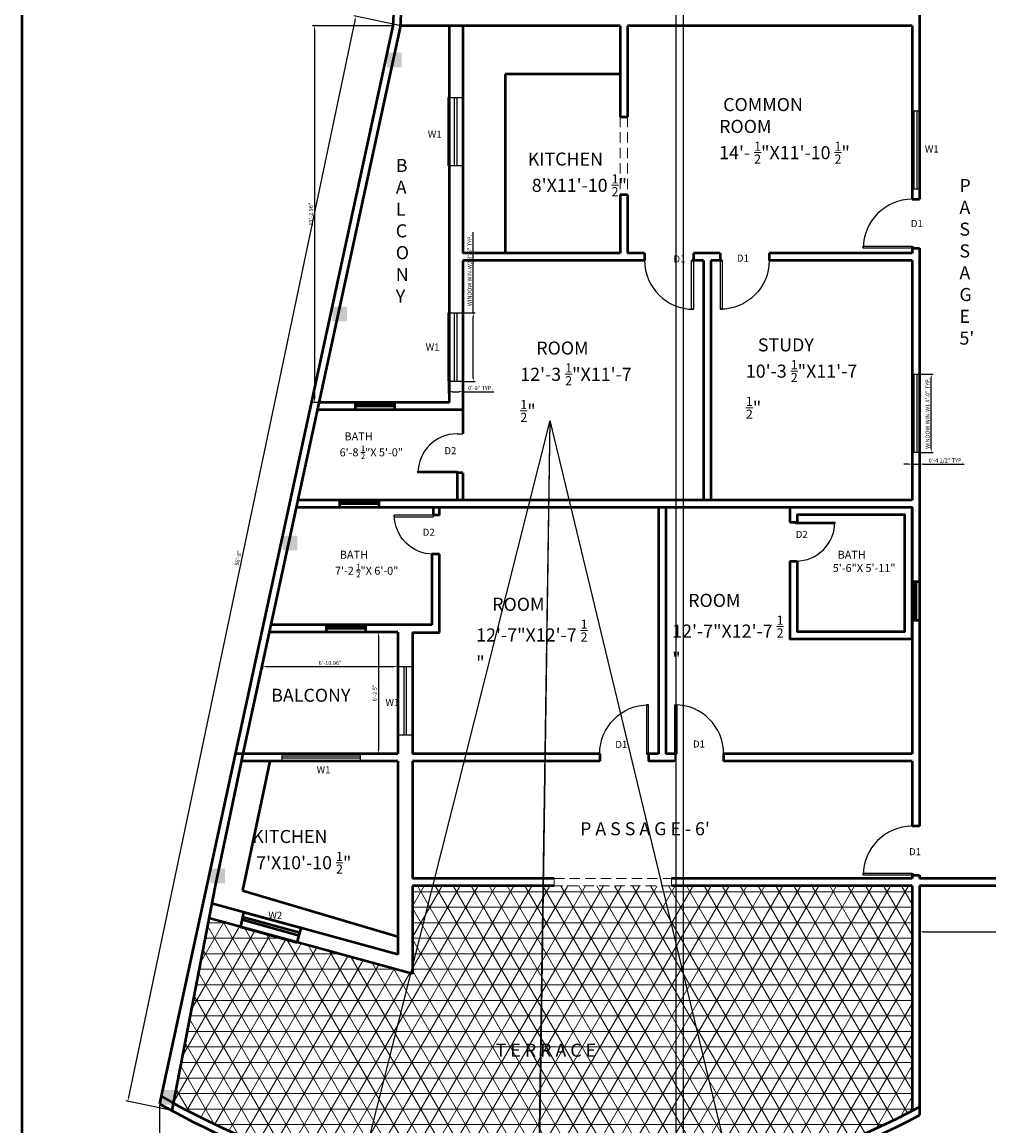
# Model space of a CAD drawing. Units: millimetres. Extents: x 1945 to 2943, y 628 to 2340.
# Tile 2 of 5: x 1945 to 2538, y 977 to 1654. Entities that reach past the tile are written whole.
import ezdxf

# ---------------------------------------------------------------- set-up
doc = ezdxf.new("R2010")
doc.units = ezdxf.units.MM
doc.linetypes.add('DASHED', pattern=[19.05, 12.7, -6.35])
for name, color, linetype, lineweight in [('A-ANNO-DIMS', 2, 'Continuous', 18), ('A-ANNO-TEXT', 7, 'Continuous', 18), ('A-AREA-IDEN', 3, 'Continuous', 18), ('A-COLS', 1, 'Continuous', 35), ('A-DOOR', 4, 'Continuous', 25), ('A-FLOR-PATT', 8, 'Continuous', 13), ('A-GLAZ', 4, 'Continuous', 25), ('A-WALL', 7, 'Continuous', 50), ('A-WALL-OPNG', 8, 'DASHED', 18)]:
    doc.layers.add(name, color=color, linetype=linetype, lineweight=lineweight)
doc.styles.get("Standard").update_dxf_attribs({"font": 'arial.ttf'})
doc.styles.add('YQ_DIM', font='SUPEROS.SHX', dxfattribs={"width": 0.8, "bigfont": 'HZDX.SHX'})
doc.dimstyles.new('ISO-25', dxfattribs={"dimtxt": 2.5, "dimasz": 2.5, "dimexe": 1.25, "dimexo": 0.625, "dimtad": 1, "dimlunit": 3, "dimtxsty": 'Standard', "dimcen": 2.5, "dimadec": 0, "dimazin": 0, "dimtfac": 1, "dimtmove": 0, "dimatfit": 3, "dimfxl": 1, "dimarcsym": 0})

# ---------------------------------------------------------------- blocks, each defined once
blk = doc.blocks.new('*U3')
for p, q in [((0, 0), (0, -6)), ((40, 0), (40, -6))]:
    blk.add_line(p, q)
blk.add_lwpolyline([(0, 0), (0, 40), (1.75, 40), (1.75, 0)], close=True)
blk.add_arc((0, 0), 40, 0, 90)
blk = doc.blocks.new('*D13')
at = {"layer": 'A-ANNO-DIMS', "color": 0, "lineweight": -2, "ltscale": 0.5, "transparency": 16777216}
for p, q in [((2092.14, 1260.11), (2092.14, 1257.27)), ((2175.1, 1260.11), (2175.1, 1257.27)), ((2094.64, 1258.52), (2172.6, 1258.52))]:
    blk.add_line(p, q, dxfattribs=at)
at = {"layer": 'A-ANNO-DIMS', "color": 0, "ltscale": 0.5, "transparency": 16777216}
for points in [[(2094.64, 1258.93), (2094.64, 1258.1), (2092.14, 1258.52)], [(2172.6, 1258.93), (2172.6, 1258.1), (2175.1, 1258.52)]]:
    blk.add_solid(points, dxfattribs=at)
at = {"layer": 'Defpoints', "color": 0, "ltscale": 0.5, "transparency": 16777216}
for p in [(2092.14, 1260.74), (2175.1, 1260.74), (2175.1, 1258.52)]:
    blk.add_point(p, dxfattribs=at)
at = {"layer": 'A-ANNO-DIMS', "color": 0, "ltscale": 0.5, "transparency": 16777216, "insert": (2133.62, 1260.42), "char_height": 2.5, "attachment_point": 5}
blk.add_mtext('6\'-10.96"', dxfattribs=at)
blk = doc.blocks.new('*D14')
at = {"layer": 'A-ANNO-DIMS', "color": 0, "lineweight": -2, "ltscale": 0.5, "transparency": 16777216}
for p, q in [((2163.22, 1277.12), (2163.22, 1207.62)), ((2163.85, 1279.62), (2164.47, 1279.62)), ((2163.85, 1205.12), (2164.47, 1205.12))]:
    blk.add_line(p, q, dxfattribs=at)
at = {"layer": 'A-ANNO-DIMS', "color": 0, "ltscale": 0.5, "transparency": 16777216}
for points in [[(2162.81, 1277.12), (2163.64, 1277.12), (2163.22, 1279.62)], [(2162.81, 1207.62), (2163.64, 1207.62), (2163.22, 1205.12)]]:
    blk.add_solid(points, dxfattribs=at)
at = {"layer": 'Defpoints', "color": 0, "ltscale": 0.5, "transparency": 16777216}
for p in [(2163.22, 1279.62), (2163.22, 1205.12), (2163.22, 1205.12)]:
    blk.add_point(p, dxfattribs=at)
at = {"layer": 'A-ANNO-DIMS', "color": 0, "ltscale": 0.5, "transparency": 16777216, "insert": (2161.32, 1242.37), "char_height": 2.5, "attachment_point": 5, "rotation": 90}
blk.add_mtext('6\'-2.5"', dxfattribs=at)
blk = doc.blocks.new('*D15')
at = {"layer": 'A-ANNO-DIMS', "color": 0, "lineweight": -2, "ltscale": 0.5, "transparency": 16777216}
for p, q in [((2171.47, 1651.58), (2122.79, 1651.58)), ((2124.04, 1649.08), (2124.04, 1423.12)), ((2126.12, 1420.62), (2122.79, 1420.62))]:
    blk.add_line(p, q, dxfattribs=at)
at = {"layer": 'A-ANNO-DIMS', "color": 0, "ltscale": 0.5, "transparency": 16777216}
for points in [[(2123.63, 1649.08), (2124.46, 1649.08), (2124.04, 1651.58)], [(2123.63, 1423.12), (2124.46, 1423.12), (2124.04, 1420.62)]]:
    blk.add_solid(points, dxfattribs=at)
at = {"layer": 'Defpoints', "color": 0, "ltscale": 0.5, "transparency": 16777216}
for p in [(2172.1, 1651.58), (2124.04, 1420.62), (2126.75, 1420.62)]:
    blk.add_point(p, dxfattribs=at)
at = {"layer": 'A-ANNO-DIMS', "color": 0, "ltscale": 0.5, "transparency": 16777216, "insert": (2122.14, 1536.1), "char_height": 2.5, "attachment_point": 5, "rotation": 90}
blk.add_mtext('19\'-2.96"', dxfattribs=at)
blk = doc.blocks.new('*D16')
at = {"layer": 'A-ANNO-DIMS', "color": 0, "lineweight": -2, "ltscale": 0.5, "transparency": 16777216}
for p, q in [((2760.6, 1123.5), (2760.6, 1094.64)), ((2495.1, 1107.96), (2495.1, 1094.64)), ((2497.6, 1095.89), (2758.1, 1095.89))]:
    blk.add_line(p, q, dxfattribs=at)
at = {"layer": 'A-ANNO-DIMS', "color": 0, "ltscale": 0.5, "transparency": 16777216}
for points in [[(2497.6, 1096.31), (2497.6, 1095.47), (2495.1, 1095.89)], [(2758.1, 1096.31), (2758.1, 1095.47), (2760.6, 1095.89)]]:
    blk.add_solid(points, dxfattribs=at)
at = {"layer": 'Defpoints', "color": 0, "ltscale": 0.5, "transparency": 16777216}
for p in [(2760.6, 1124.12), (2495.1, 1108.59), (2760.6, 1095.89)]:
    blk.add_point(p, dxfattribs=at)
at = {"layer": 'A-ANNO-DIMS', "color": 0, "ltscale": 0.5, "transparency": 16777216, "insert": (2627.85, 1097.79), "char_height": 2.5, "attachment_point": 5}
blk.add_mtext('22\'-1.5"', dxfattribs=at)
blk = doc.blocks.new('*D10')
at = {"layer": 'A-ANNO-DIMS', "color": 0, "lineweight": -2, "ltscale": 0.5, "transparency": 16777216}
for p, q in [((2148.79, 1654.96), (2010, 994.38)), ((2176.25, 1651.75), (2148.08, 1657.67)), ((2036.43, 986.28), (2008.27, 992.19))]:
    blk.add_line(p, q, dxfattribs=at)
at = {"layer": 'A-ANNO-DIMS', "color": 0, "ltscale": 0.5, "transparency": 16777216}
for points in [[(2148.39, 1655.05), (2149.2, 1654.88), (2149.31, 1657.41)], [(2009.6, 994.47), (2010.41, 994.3), (2009.49, 991.94)]]:
    blk.add_solid(points, dxfattribs=at)
at = {"layer": 'Defpoints', "color": 0, "ltscale": 0.5, "transparency": 16777216}
for p in [(2176.86, 1651.62), (2009.49, 991.94), (2037.04, 986.15)]:
    blk.add_point(p, dxfattribs=at)
at = {"layer": 'A-ANNO-DIMS', "color": 0, "ltscale": 0.5, "transparency": 16777216, "insert": (2077.54, 1325.06), "char_height": 2.5, "attachment_point": 5, "rotation": 78.13463}
blk.add_mtext('56\'-8"', dxfattribs=at)
blk = doc.blocks.new('WIN-W1')
for points in [[(0, 48), (4.5, 48), (4.5, 0), (0, 0)], [(1.29, 48), (2.82, 48), (2.82, 0), (1.29, 0)]]:
    blk.add_lwpolyline(points, close=True)
blk = doc.blocks.new('WIN-W2')
for points in [[(0, 42), (9, 42), (9, 0), (0, 0)], [(3.84, 42), (5.13, 42), (5.13, 0), (3.84, 0)]]:
    blk.add_lwpolyline(points, close=True)
blk = doc.blocks.new('*D20')
at = {"layer": 'A-ANNO-DIMS', "color": 0, "lineweight": -2, "transparency": 16777216}
for p, q in [((2495.72, 1437.94), (2503.55, 1437.94)), ((2502.3, 1392.44), (2502.3, 1435.44)), ((2495.72, 1389.94), (2503.55, 1389.94))]:
    blk.add_line(p, q, dxfattribs=at)
at = {"layer": 'A-ANNO-DIMS', "color": 0, "transparency": 16777216}
for points in [[(2501.88, 1435.44), (2502.71, 1435.44), (2502.3, 1437.94)], [(2501.88, 1392.44), (2502.71, 1392.44), (2502.3, 1389.94)]]:
    blk.add_solid(points, dxfattribs=at)
at = {"layer": 'Defpoints', "color": 0, "transparency": 16777216}
for p in [(2495.1, 1437.94), (2502.3, 1437.94), (2495.1, 1389.94)]:
    blk.add_point(p, dxfattribs=at)
at = {"layer": 'A-ANNO-DIMS', "color": 0, "transparency": 16777216, "insert": (2500.38, 1413.94), "char_height": 2.5, "attachment_point": 5, "rotation": 90}
blk.add_mtext('WINDOW WIN-W1 4\'-0" TYP.', dxfattribs=at)
blk = doc.blocks.new('*D21')
at = {"layer": 'A-ANNO-DIMS', "color": 0, "lineweight": -2, "transparency": 16777216}
for p, q in [((2490.6, 1389.32), (2490.6, 1381.49)), ((2495.1, 1389.32), (2495.1, 1381.49)), ((2488.1, 1382.74), (2485.6, 1382.74)), ((2490.6, 1382.74), (2495.1, 1382.74)), ((2497.6, 1382.74), (2522.41, 1382.74))]:
    blk.add_line(p, q, dxfattribs=at)
at = {"layer": 'A-ANNO-DIMS', "color": 0, "transparency": 16777216}
for points in [[(2488.1, 1383.16), (2488.1, 1382.32), (2490.6, 1382.74)], [(2497.6, 1383.16), (2497.6, 1382.32), (2495.1, 1382.74)]]:
    blk.add_solid(points, dxfattribs=at)
at = {"layer": 'Defpoints', "color": 0, "transparency": 16777216}
for p in [(2490.6, 1389.94), (2495.1, 1389.94), (2495.1, 1382.74)]:
    blk.add_point(p, dxfattribs=at)
at = {"layer": 'A-ANNO-DIMS', "color": 0, "transparency": 16777216, "insert": (2511.25, 1384.66), "char_height": 2.5, "attachment_point": 5}
blk.add_mtext('0\'-4 1/2" TYP.', dxfattribs=at)
blk = doc.blocks.new('*D22')
at = {"layer": 'A-ANNO-DIMS', "color": 0, "lineweight": -2, "transparency": 16777216}
for p, q in [((2221.4, 1475.48), (2221.4, 1525.03)), ((2215.72, 1475.48), (2222.65, 1475.48)), ((2221.4, 1435.98), (2221.4, 1472.98)), ((2215.72, 1433.48), (2222.65, 1433.48))]:
    blk.add_line(p, q, dxfattribs=at)
at = {"layer": 'A-ANNO-DIMS', "color": 0, "transparency": 16777216}
for points in [[(2220.98, 1472.98), (2221.81, 1472.98), (2221.4, 1475.48)], [(2220.98, 1435.98), (2221.81, 1435.98), (2221.4, 1433.48)]]:
    blk.add_solid(points, dxfattribs=at)
at = {"layer": 'Defpoints', "color": 0, "transparency": 16777216}
for p in [(2215.1, 1475.48), (2221.4, 1475.48), (2215.1, 1433.48)]:
    blk.add_point(p, dxfattribs=at)
at = {"layer": 'A-ANNO-DIMS', "color": 0, "transparency": 16777216, "insert": (2219.48, 1501.5), "char_height": 2.5, "attachment_point": 5, "rotation": 90}
blk.add_mtext('WINDOW WIN-W2 3\'-6" TYP.', dxfattribs=at)
blk = doc.blocks.new('*D23')
at = {"layer": 'A-ANNO-DIMS', "color": 0, "lineweight": -2, "transparency": 16777216}
for p, q in [((2206.1, 1432.86), (2206.1, 1425.93)), ((2215.1, 1432.86), (2215.1, 1425.93)), ((2208.6, 1427.18), (2212.6, 1427.18)), ((2215.1, 1427.18), (2234.09, 1427.18))]:
    blk.add_line(p, q, dxfattribs=at)
at = {"layer": 'A-ANNO-DIMS', "color": 0, "transparency": 16777216}
for points in [[(2208.6, 1427.6), (2208.6, 1426.76), (2206.1, 1427.18)], [(2212.6, 1427.6), (2212.6, 1426.76), (2215.1, 1427.18)]]:
    blk.add_solid(points, dxfattribs=at)
at = {"layer": 'Defpoints', "color": 0, "transparency": 16777216}
for p in [(2206.1, 1433.48), (2215.1, 1433.48), (2215.1, 1427.18)]:
    blk.add_point(p, dxfattribs=at)
at = {"layer": 'A-ANNO-DIMS', "color": 0, "transparency": 16777216, "insert": (2225.84, 1429.08), "char_height": 2.5, "attachment_point": 5}
blk.add_mtext('0\'-9" TYP.', dxfattribs=at)
blk = doc.blocks.new('*D24')
at = {"layer": 'A-ANNO-DIMS', "color": 0, "lineweight": -2, "transparency": 16777216}
for p, q in [((2760.6, 1123.5), (2760.6, 857.56)), ((2029.02, 989.8), (2029.02, 857.56)), ((2031.52, 858.81), (2758.1, 858.81))]:
    blk.add_line(p, q, dxfattribs=at)
at = {"layer": 'A-ANNO-DIMS', "color": 0, "transparency": 16777216}
for points in [[(2031.52, 859.23), (2031.52, 858.39), (2029.02, 858.81)], [(2758.1, 859.23), (2758.1, 858.39), (2760.6, 858.81)]]:
    blk.add_solid(points, dxfattribs=at)
at = {"layer": 'Defpoints', "color": 0, "transparency": 16777216}
for p in [(2760.6, 1124.12), (2029.02, 990.43), (2760.6, 858.81)]:
    blk.add_point(p, dxfattribs=at)
at = {"layer": 'A-ANNO-DIMS', "color": 0, "transparency": 16777216, "insert": (2394.81, 860.73), "char_height": 2.5, "attachment_point": 5}
blk.add_mtext('60\'-11 1/2"', dxfattribs=at)
blk = doc.blocks.new('*D25')
at = {"layer": 'A-ANNO-DIMS', "color": 0, "lineweight": -2, "transparency": 16777216}
for p, q in [((2268.43, 1409.46), (2261.15, 926.91)), ((2256.65, 628.35), (2261.11, 924.41))]:
    blk.add_line(p, q, dxfattribs=at)
at = {"layer": 'A-ANNO-DIMS', "color": 0, "transparency": 16777216}
blk.add_solid([(2260.7, 924.42), (2261.53, 924.4), (2261.15, 926.91)], dxfattribs=at)
at = {"layer": 'Defpoints', "color": 0, "transparency": 16777216}
for p in [(2268.43, 1409.46), (2261.15, 926.91)]:
    blk.add_point(p, dxfattribs=at)
at = {"layer": 'A-ANNO-DIMS', "color": 0, "transparency": 16777216, "insert": (2254.87, 637.41), "char_height": 2.5, "attachment_point": 5, "rotation": 89.13551}
blk.add_mtext('R40\'-2 1/2"', dxfattribs=at)
blk = doc.blocks.new('*D26')
at = {"layer": 'A-ANNO-DIMS', "color": 0, "lineweight": -2, "transparency": 16777216}
for p, q in [((2268.43, 1409.46), (2261.71, 931.4)), ((2257.57, 637.48), (2261.67, 928.9))]:
    blk.add_line(p, q, dxfattribs=at)
at = {"layer": 'A-ANNO-DIMS', "color": 0, "transparency": 16777216}
blk.add_solid([(2261.26, 928.91), (2262.09, 928.9), (2261.71, 931.4)], dxfattribs=at)
at = {"layer": 'Defpoints', "color": 0, "transparency": 16777216}
for p in [(2268.43, 1409.46), (2261.71, 931.4)]:
    blk.add_point(p, dxfattribs=at)
at = {"layer": 'A-ANNO-DIMS', "color": 0, "transparency": 16777216, "insert": (2255.77, 644.6), "char_height": 2.5, "attachment_point": 5, "rotation": 89.19401}
blk.add_mtext('R39\'-10"', dxfattribs=at)
blk = doc.blocks.new('*D30')
at = {"layer": 'A-ANNO-DIMS', "color": 0, "lineweight": -2, "transparency": 16777216}
for p, q in [((2345.6, 2086), (2345.6, 856.56)), ((2350.1, 2086), (2350.1, 856.56)), ((2343.1, 857.81), (2340.6, 857.81)), ((2345.6, 857.81), (2350.1, 857.81)), ((2352.6, 857.81), (2368.82, 857.81))]:
    blk.add_line(p, q, dxfattribs=at)
at = {"layer": 'A-ANNO-DIMS', "color": 0, "transparency": 16777216}
for points in [[(2343.1, 858.23), (2343.1, 857.39), (2345.6, 857.81)], [(2352.6, 858.23), (2352.6, 857.39), (2350.1, 857.81)]]:
    blk.add_solid(points, dxfattribs=at)
at = {"layer": 'Defpoints', "color": 0, "transparency": 16777216}
for p in [(2345.6, 2086.62), (2350.1, 2086.62), (2350.1, 857.81)]:
    blk.add_point(p, dxfattribs=at)
at = {"layer": 'A-ANNO-DIMS', "color": 0, "transparency": 16777216, "insert": (2361.96, 859.73), "char_height": 2.5, "attachment_point": 5}
blk.add_mtext('0\'-4 1/2"', dxfattribs=at)
blk = doc.blocks.new('*D31')
at = {"layer": 'A-ANNO-DIMS', "color": 0, "lineweight": -2, "transparency": 16777216}
for p, q in [((2268.43, 1409.46), (2150.43, 941.5)), ((2077.42, 651.98), (2149.82, 939.08))]:
    blk.add_line(p, q, dxfattribs=at)
at = {"layer": 'A-ANNO-DIMS', "color": 0, "transparency": 16777216}
blk.add_solid([(2149.41, 939.18), (2150.22, 938.98), (2150.43, 941.5)], dxfattribs=at)
at = {"layer": 'Defpoints', "color": 0, "transparency": 16777216}
for p in [(2268.43, 1409.46), (2150.43, 941.5)]:
    blk.add_point(p, dxfattribs=at)
at = {"layer": 'A-ANNO-DIMS', "color": 0, "transparency": 16777216, "insert": (2077.77, 661.2), "char_height": 2.5, "attachment_point": 5, "rotation": 75.84677}
blk.add_mtext('R40\'-2 1/2"', dxfattribs=at)
blk = doc.blocks.new('*D32')
at = {"layer": 'A-ANNO-DIMS', "color": 0, "lineweight": -2, "transparency": 16777216}
for p, q in [((2268.43, 1409.46), (2380.4, 944.65)), ((2449.24, 658.88), (2380.98, 942.22))]:
    blk.add_line(p, q, dxfattribs=at)
at = {"layer": 'A-ANNO-DIMS', "color": 0, "transparency": 16777216}
blk.add_solid([(2381.39, 942.32), (2380.58, 942.12), (2380.4, 944.65)], dxfattribs=at)
at = {"layer": 'Defpoints', "color": 0, "transparency": 16777216}
for p in [(2268.43, 1409.46), (2380.4, 944.65)]:
    blk.add_point(p, dxfattribs=at)
at = {"layer": 'A-ANNO-DIMS', "color": 0, "transparency": 16777216, "insert": (2449.43, 666.21), "char_height": 2.5, "attachment_point": 5, "rotation": 283.5436}
blk.add_mtext('R39\'-10"', dxfattribs=at)

msp = doc.modelspace()

# ---------------------------------------------------------------- hatches: boundary and pattern name
at = {"layer": 'A-COLS'}
h = msp.add_hatch(color=256, dxfattribs=at)
h.dxf.hatch_style = 1
h.paths.add_polyline_path([(2177.484, 1635.09), (2168.484, 1635.09), (2168.484, 1626.09), (2177.484, 1626.09)])
h = msp.add_hatch(color=256, dxfattribs=at)
h.dxf.hatch_style = 1
h.paths.add_polyline_path([(2144.054, 1479.377), (2135.054, 1479.377), (2135.054, 1470.377), (2144.054, 1470.377)])
h = msp.add_hatch(color=256, dxfattribs=at)
h.dxf.hatch_style = 1
h.paths.add_polyline_path([(2113.425, 1338.927), (2104.425, 1338.927), (2104.425, 1329.927), (2113.425, 1329.927)])
h = msp.add_hatch(color=256, dxfattribs=at)
h.dxf.hatch_style = 1
h.paths.add_polyline_path([(2069.161, 1134.642), (2060.161, 1134.642), (2060.161, 1125.642), (2069.161, 1125.642)])
h = msp.add_hatch(color=256, dxfattribs=at)
h.dxf.hatch_style = 1
h.paths.add_polyline_path([(2038.7, 998.916), (2029.7, 998.916), (2029.7, 989.916), (2038.7, 989.916)])
at = {"layer": 'A-FLOR-PATT'}
h = msp.add_hatch(dxfattribs=at)
h.set_pattern_fill('NET3', color=256, scale=3)
h.set_pattern_definition([(0, (1094.862, 577.549), (0, 9.525), []), (60, (1094.862, 577.549), (-8.24889, 4.7625), []), (120, (1094.862, 577.549), (-8.24889, -4.7625), [])])
h.paths.add_polyline_path([(2490.597, 1124.121), (2184.097, 1124.121), (2184.097, 1070.121), (2059.269, 1104.268), (2037.334, 990.918, 0.252088), (2490.597, 986.107)])

# ---------------------------------------------------------------- linework, layer by layer
at = {"layer": 'A-WALL'}
for p, q in [((2203.597, 2252.621), (2172.098, 1651.581)), ((2208.091, 2252.386), (2176.56, 1650.732)), ((2495.097, 1660.225), (2495.097, 1545.177)), ((2172.162, 1651.684), (2029.018, 990.428)), ((2176.56, 1650.732), (2080.097, 1205.121)), ((2311.597, 1651.621), (2176.859, 1651.621)), ((2206.597, 1651.621), (2206.597, 1420.622)), ((2215.097, 1651.621), (2215.097, 1512.121)), ((2311.597, 1651.621), (2311.597, 1595.88)), ((2490.597, 1651.621), (2316.097, 1651.621)), ((2316.097, 1651.621), (2316.097, 1595.88)), ((2490.597, 1651.621), (2490.597, 1545.177)), ((2311.597, 1621.988), (2241.043, 1621.988)), ((2241.043, 1621.988), (2241.043, 1512.121)), ((2311.597, 1547.88), (2311.597, 1512.121)), ((2316.097, 1547.88), (2316.097, 1512.121)), ((2490.597, 1545.177), (2495.097, 1545.177)), ((2311.597, 1512.121), (2215.097, 1512.121)), ((2326.536, 1512.121), (2316.097, 1512.121)), ((2326.536, 1512.121), (2326.536, 1507.621)), ((2372.854, 1512.121), (2356.469, 1512.121)), ((2356.469, 1512.121), (2356.469, 1507.621)), ((2372.854, 1512.121), (2372.854, 1507.621)), ((2490.597, 1512.121), (2402.922, 1512.121)), ((2402.922, 1512.121), (2402.922, 1507.705)), ((2490.597, 1516.49), (2490.597, 1512.121)), ((2490.597, 1515.177), (2495.097, 1515.177)), ((2495.097, 1515.177), (2495.097, 1160.592)), ((2326.536, 1507.621), (2215.097, 1507.621)), ((2215.097, 1507.621), (2215.097, 1401.341)), ((2362.597, 1507.621), (2355.419, 1507.621)), ((2362.597, 1507.621), (2362.597, 1360.621)), ((2373.904, 1507.621), (2367.097, 1507.621)), ((2367.097, 1507.621), (2367.097, 1360.621)), ((2490.597, 1507.621), (2402.921, 1507.621)), ((2490.597, 1507.621), (2490.597, 1360.621)), ((2206.597, 1420.622), (2126.748, 1420.624)), ((2215.097, 1416.121), (2126.748, 1416.124)), ((2215.097, 1377.341), (2211.497, 1377.341)), ((2211.497, 1377.341), (2211.497, 1360.621)), ((2215.097, 1377.341), (2215.097, 1360.621)), ((2184.097, 1356.121), (2112.785, 1356.121)), ((2490.597, 1360.621), (2113.759, 1360.621)), ((2490.597, 1356.121), (2184.097, 1356.121)), ((2196.979, 1351.507), (2196.979, 1356.121)), ((2200.694, 1351.507), (2200.694, 1356.121)), ((2335.097, 1356.121), (2335.097, 1205.121)), ((2339.597, 1356.121), (2339.597, 1205.121)), ((2490.597, 1356.121), (2490.597, 1205.121)), ((2200.694, 1351.507), (2196.979, 1351.507)), ((2415.597, 1347.247), (2420.097, 1347.247)), ((2196.079, 1327.524), (2196.079, 1284.121)), ((2200.694, 1327.507), (2196.079, 1327.507)), ((2200.694, 1279.457), (2200.694, 1327.507)), ((2415.597, 1323.247), (2420.097, 1323.247)), ((2196.079, 1284.121), (2097.199, 1284.121)), ((2175.097, 1279.621), (2096.225, 1279.621)), ((2175.097, 1279.621), (2175.097, 1205.121)), ((2184.097, 1279.457), (2184.097, 1205.121)), ((2184.097, 1279.457), (2196.079, 1279.457)), ((2196.079, 1279.457), (2200.694, 1279.457)), ((2080.097, 1205.121), (2063.111, 1124.121)), ((2175.097, 1205.121), (2075.493, 1205.121)), ((2175.097, 1200.621), (2079.154, 1200.621)), ((2175.097, 1200.621), (2175.097, 1128.621)), ((2175.097, 1200.621), (2175.097, 1081.914)), ((2298.979, 1205.121), (2184.097, 1205.121)), ((2298.979, 1200.621), (2184.097, 1200.621)), ((2184.097, 1200.621), (2184.097, 1128.621)), ((2298.979, 1205.121), (2298.979, 1200.621)), ((2335.097, 1205.121), (2327.929, 1205.121)), ((2328.979, 1205.121), (2328.979, 1200.621)), ((2344.987, 1200.621), (2328.979, 1200.621)), ((2346.299, 1205.121), (2339.597, 1205.121)), ((2490.597, 1205.121), (2374.987, 1205.121)), ((2374.987, 1205.121), (2374.987, 1200.621)), ((2490.597, 1200.621), (2374.987, 1200.621)), ((2490.597, 1200.621), (2490.597, 1160.592)), ((2495.097, 1160.592), (2490.597, 1160.592)), ((2490.597, 1131.904), (2490.597, 1128.621)), ((2063.111, 1124.121), (2036.436, 986.276)), ((2175.097, 1124.121), (2175.097, 1081.914)), ((2270.98, 1128.621), (2184.097, 1128.621)), ((2270.98, 1124.121), (2184.097, 1124.121)), ((2184.097, 1124.121), (2184.097, 1070.121)), ((2490.597, 1128.621), (2342.98, 1128.621)), ((2490.597, 1124.121), (2342.98, 1124.121)), ((2490.597, 1130.592), (2495.097, 1130.592)), ((2490.597, 1124.121), (2490.597, 986.107)), ((2495.097, 1130.592), (2495.097, 1128.621)), ((2548.097, 1128.621), (2495.097, 1128.621)), ((2760.597, 1124.121), (2495.097, 1124.121)), ((2495.097, 1124.121), (2495.097, 983.395)), ((2175.097, 1081.914), (2061.644, 1112.949)), ((2184.097, 1070.121), (2059.269, 1104.268))]:
    msp.add_line(p, q, dxfattribs=at)
at = {"layer": 'A-WALL', "ltscale": 0.5}
for p, q in [((2311.597, 1595.88), (2316.097, 1595.88)), ((2316.097, 1547.88), (2311.597, 1547.88)), ((2096.7, 1200.621), (2079.889, 1121.137)), ((2079.889, 1121.137), (2175.097, 1092.939)), ((2080.53, 1107.783), (2078.666, 1098.962)), ((2114.959, 1095.2), (2079.914, 1104.867)), ((2115.764, 1098.144), (2080.53, 1107.783)), ((2078.666, 1098.962), (2113.322, 1089.217)), ((2079.598, 1103.372), (2114.543, 1093.68)), ((2113.322, 1089.217), (2115.764, 1098.144)), ((2114.543, 1093.68), (2114.959, 1095.2))]:
    msp.add_line(p, q, dxfattribs=at)
for points in [[(1944.667, 2340.145), (2943.065, 2340.145), (2943.065, 839.363), (1944.667, 839.363)], [(2173.145, 1420.623), (2173.145, 1416.123), (2149.145, 1416.123), (2149.145, 1420.623)], [(2173.145, 1419.236), (2173.145, 1418.373), (2149.145, 1418.373), (2149.145, 1419.236)], [(2163.497, 1360.621), (2163.497, 1356.121), (2139.497, 1356.121), (2139.497, 1360.621)], [(2163.497, 1359.235), (2163.497, 1358.371), (2139.497, 1358.371), (2139.497, 1359.235)], [(2490.597, 1310.791), (2495.097, 1310.791), (2495.097, 1286.791), (2490.597, 1286.791)], [(2491.984, 1310.791), (2492.847, 1310.791), (2492.847, 1286.791), (2491.984, 1286.791)], [(2155.4, 1284.121), (2155.4, 1279.621), (2131.4, 1279.621), (2131.4, 1284.121)], [(2155.4, 1282.735), (2155.4, 1281.871), (2131.4, 1281.871), (2131.4, 1282.735)]]:
    msp.add_lwpolyline(points, close=True, dxfattribs=at)
at = {"layer": 'A-WALL'}
for points in [[(2415.597, 1323.247), (2415.597, 1275.621), (2490.597, 1275.621), (2490.597, 1356.121), (2415.597, 1356.121), (2415.597, 1347.247)], [(2420.097, 1323.263), (2420.097, 1280.121), (2486.097, 1280.121), (2486.097, 1351.621), (2420.097, 1351.621), (2420.097, 1346.197)]]:
    msp.add_lwpolyline(points, dxfattribs=at)
for radius, start, end in [(482.602, 240.258112, 298.012953), (478.102, 240.087713, 298.300235)]:
    msp.add_arc((2268.433, 1409.456), radius, start, end, dxfattribs=at)
at = {"layer": 'A-WALL-OPNG', "ltscale": 0.5}
for p, q in [((2311.597, 1595.88), (2311.597, 1547.88)), ((2316.097, 1595.88), (2316.097, 1547.88)), ((2270.98, 1128.621), (2270.98, 1124.121)), ((2270.98, 1128.621), (2342.98, 1128.621)), ((2342.98, 1124.121), (2270.98, 1124.121)), ((2342.98, 1128.621), (2342.98, 1124.121))]:
    msp.add_line(p, q, dxfattribs=at)

# ---------------------------------------------------------------- block references
at = {"layer": 'A-DOOR'}
for p, xscale, yscale, zscale, rotation in [((2490.597, 1515.177), 0.75, 0.75, 0.75, 90.00000000000003), ((2356.536, 1507.705), 0.75, 0.75, 0.75, 180), ((2372.922, 1507.705), -0.75, 0.75, 0.75, 180), ((2211.497, 1377.341), 0.6, 0.6, 0.6, 90), ((2196.979, 1351.507), -0.6, 0.6, 0.6, 90), ((2419.197, 1347.247), 0.6, 0.6, 0.6, 270), ((2490.597, 1130.592), 0.75, 0.75, 0.75, 90.00000000000003)]:
    msp.add_blockref('*U3', p, dxfattribs=dict(at, xscale=xscale, yscale=yscale, zscale=zscale, rotation=rotation))
at = {"layer": 'A-DOOR', "yscale": 0.75, "zscale": 0.75}
for p, xscale in [((2328.979, 1205.121), -0.75), ((2344.987, 1205.121), 0.75)]:
    msp.add_blockref('*U3', p, dxfattribs=dict(at, xscale=xscale))
at = {"layer": 'A-GLAZ'}
for name, p in [('WIN-W2', (2206.097, 1565.729)), ('WIN-W1', (2490.597, 1551.379)), ('WIN-W2', (2206.097, 1433.481)), ('WIN-W1', (2490.597, 1389.94)), ('WIN-W2', (2175.097, 1216.516))]:
    msp.add_blockref(name, p, dxfattribs=at)
at = {"layer": 'A-GLAZ', "rotation": 270.0000000000001}
msp.add_blockref('WIN-W1', (2104.112, 1205.122), dxfattribs=at)

# ---------------------------------------------------------------- texts
at = {"layer": 'A-ANNO-TEXT', "ltscale": 0.5, "char_height": 4.35068, "attachment_point": 1, "style": 'YQ_DIM'}
for s, insert in [('{\\f@Arial Unicode MS|b0|i0|c0|p34;W1}', (2193.549, 1587.278)), ('{\\f@Arial Unicode MS|b0|i0|c0|p34;W1}', (2498.384, 1578.249)), ('{\\f@Arial Unicode MS|b0|i0|c0|p34;D1}', (2489.793, 1532.46)), ('{\\f@Arial Unicode MS|b0|i0|c0|p34;D1}', (2344.185, 1510.793)), ('{\\f@Arial Unicode MS|b0|i0|c0|p34;D1}', (2383.087, 1511.273)), ('{\\f@Arial Unicode MS|b0|i0|c0|p34;W1}', (2192.222, 1456.749)), ('{\\f@Arial Unicode MS|b0|i0|c0|p34;D2}', (2203.667, 1393.182)), ('{\\f@Arial Unicode MS|b0|i0|c0|p34;D2}', (2190.401, 1343.13)), ('{\\f@Arial Unicode MS|b0|i0|c0|p34;D2}', (2419.187, 1341.812)), ('{\\f@Arial Unicode MS|b0|i0|c0|p34;W1}', (2167.563, 1238.772)), ('{\\f@Arial Unicode MS|b0|i0|c0|p34;D1}', (2308.519, 1212.987)), ('{\\f@Arial Unicode MS|b0|i0|c0|p34;D1}', (2356.177, 1213.236)), ('{\\f@Arial Unicode MS|b0|i0|c0|p34;W1}', (2125.333, 1197.475)), ('{\\f@Arial Unicode MS|b0|i0|c0|p34;D1}', (2488.72, 1147.204)), ('{\\f@Arial Unicode MS|b0|i0|c0|p34;W2}', (2095.717, 1108.206))]:
    msp.add_mtext_dynamic_manual_height_columns(s, width=7.90712, gutter_width=21.753, heights=[0], dxfattribs=dict(at, insert=insert))
at = {"layer": 'A-AREA-IDEN', "ltscale": 0.5, "attachment_point": 1, "style": 'YQ_DIM'}
for s, width, gutter_width, heights, insert, char_height in [('\\A1;{\\f@Malgun Gothic|b0|i0|c0|p34; COMMON  ROOM \\P14\'- \\H0.7x;\\S1/2;\\H1.42857x;"X11\'-10 \\H0.7x;\\S1/2;\\H1.42857x;"}', 88.00213, 40.122, [0], (2372.218, 1607.31), 8.02448), ('\\A1; {\\fMicrosoft YaHei UI|b0|i0|c0|p34;KITCHEN\\P  8\'X11\'-10 \\H0.7x;\\S1/2;\\H1.42857x;"}', 67.57438, 12.5, [43.34], (2252.393, 1573.881), 8.02), ('{\\fAcadEref|b0|i0|c0|p2;B\\f@Arial Unicode MS|b1|i1|c0|p34; A\\PL\\PC\\PO\\PN\\PY}', 12.11312, 12.5, [99.959], (2173.872, 1569.959), 8.02), ("{\\f@Arial Unicode MS|b0|i0|c0|p34;P\\PA\\PS\\PS\\PA\\PG\\PE\\P5'}", 12.11312, 12.5, [123.216], (2519.598, 1557.635), 8.02), ('\\A1;{\\f@Malgun Gothic|b0|i0|c0|p34;    ROOM \\P12\'-3 \\H0.7x;\\S1/2;\\H1.42857x;"X11\'-7 \\H0.7x;\\S1/2;\\H1.42857x;"}', 69.89446, 40.122, [0], (2250.248, 1457.955), 8.02448), ('\\A1;{\\f@Malgun Gothic|b0|i0|c0|p34;   STUDY\\P10\'-3 \\H0.7x;\\S1/2;\\H1.42857x;"X11\'-7 \\H0.7x;\\S1/2;\\H1.42857x;"}', 69.89446, 40.122, [0], (2388.607, 1459.904), 8.02448), ('\\A1;{  \\fSegoe UI Black|b0|i0|c0|p34;BATH\\P6\'-8 \\H0.7x;\\S1/2;\\H1.42857x;"X 5\'-0"}', 43.60909, 24.448, [0], (2139.424, 1402.235), 4.88966), ('\\A1;{  \\fSegoe UI Black|b0|i0|c0|p34;BATH\\P7\'-2 \\H0.7x;\\S1/2;\\H1.42857x;"X 6\'-0"}', 43.60909, 24.448, [0], (2136.581, 1329.62), 4.88966), ('\\A1;{  \\fSegoe UI Black|b0|i0|c0|p34;BATH\\P5\'-6\\H1x;"X 5\'-11"}', 43.60909, 24.448, [0], (2441.911, 1329.62), 4.88966), ('\\A1;{\\f@Malgun Gothic|b0|i0|c0|p34;    ROOM \\P12\'-7\\H1x;"X12\'-7 \\H0.7x;\\S1/2;\\H1.42857x;"}', 69.89446, 40.122, [0], (2223.212, 1300.793), 8.02448), ('\\A1;{\\f@Malgun Gothic|b0|i0|c0|p34;    ROOM \\P12\'-7\\H1x;"X12\'-7 \\H0.7x;\\S1/2;\\H1.42857x;"}', 69.89446, 40.122, [0], (2343.421, 1303.18), 8.02448), ('\\A1;{\\fGabriola|b0|i0|c0|p82;BALCONY}', 67.57438, 12.5, [14.95], (2097.464, 1244.983), 8.02), ('\\A1; {\\fMicrosoft YaHei UI|b0|i0|c0|p34;KITCHEN\\P  7\'X10\'-10 \\H0.7x;\\S1/2;\\H1.42857x;"}', 67.57438, 12.5, [43.34], (2083.362, 1158.347), 8.02), ('{\\f@Arial Unicode MS|b0|i0|c0|p34;T E R R A C E}', 108.12884, 12.5, [1.216], (2235.137, 1027.241), 8.02)]:
    msp.add_mtext_dynamic_manual_height_columns(s, width=width, gutter_width=gutter_width, heights=heights, dxfattribs=dict(at, insert=insert, char_height=char_height))
at = {"layer": 'A-AREA-IDEN', "insert": (2326.732, 1159.085), "char_height": 8, "attachment_point": 5, "style": 'YQ_DIM'}
msp.add_mtext_dynamic_manual_height_columns("{\\f@MS PGothic|b0|i0|c0|p34;P A S S A G E - 6'}", width=111.08232, gutter_width=12.5, heights=[0], dxfattribs=at)

# ---------------------------------------------------------------- dimensions: what is measured, and where the dimension line sits
at = {"layer": 'A-ANNO-DIMS'}
for base, p1, p2, picture, middle in [((2350.097, 857.809), (2345.597, 2086.621), (2350.097, 2086.621), '*D30', (2361.958, 859.727)), ((2760.597, 858.809), (2029.018, 990.428), (2760.597, 1124.121), '*D24', (2394.808, 860.727))]:
    dim = msp.add_linear_dim(base=base, p1=p1, p2=p2, dimstyle='ISO-25', override={"dimdec": 1, "dimlfac": 1, "dimrnd": 0, "dimzin": 1, "dimdsep": 46, "dimlunit": 4, "dimfrac": 2}, dxfattribs=at)
    dim.commit()
    dim.dimension.update_dxf_attribs({"geometry": picture, "text_midpoint": middle})
at = {"layer": 'A-ANNO-DIMS', "ltscale": 0.5}
dim = msp.add_aligned_dim(p1=(2176.859, 1651.621), p2=(2037.041, 986.148), distance=-28.153, dimstyle='ISO-25', override={"dimclrd": 0, "dimclre": 0, "dimclrt": 0}, dxfattribs=at)
dim.commit()
dim.dimension.update_dxf_attribs({"geometry": '*D10', "text_midpoint": (2077.538, 1325.064)})
for base, p1, p2, picture, middle in [((2124.043, 1420.624), (2172.098, 1651.581), (2126.748, 1420.624), '*D15', (2122.141, 1536.102)), ((2163.225, 1205.121), (2163.225, 1279.621), (2163.225, 1205.121), '*D14', (2161.323, 1242.371))]:
    dim = msp.add_linear_dim(base=base, p1=p1, p2=p2, angle=90, dimstyle='ISO-25', override={"dimclrd": 0, "dimclre": 0, "dimclrt": 0}, dxfattribs=at)
    dim.commit()
    dim.dimension.update_dxf_attribs({"geometry": picture, "text_midpoint": middle})
at = {"layer": 'A-ANNO-DIMS'}
for base, p1, p2, text, picture, middle in [((2221.397, 1475.481), (2215.097, 1433.481), (2215.097, 1475.481), 'WINDOW WIN-W2 <> TYP.', '*D22', (2219.478, 1501.504)), ((2502.297, 1437.94), (2495.097, 1389.94), (2495.097, 1437.94), 'WINDOW WIN-W1 <> TYP.', '*D20', (2500.379, 1413.94))]:
    dim = msp.add_linear_dim(base=base, p1=p1, p2=p2, angle=90, text=text, dimstyle='ISO-25', override={"dimdec": 1, "dimrnd": 0, "dimzin": 1, "dimlunit": 4, "dimfrac": 2}, dxfattribs=at)
    dim.commit()
    dim.dimension.update_dxf_attribs({"geometry": picture, "text_midpoint": middle})
for base, p1, p2, picture, middle in [((2215.097, 1427.181), (2206.097, 1433.481), (2215.097, 1433.481), '*D23', (2225.842, 1429.083)), ((2495.097, 1382.74), (2490.597, 1389.94), (2495.097, 1389.94), '*D21', (2511.254, 1384.658))]:
    dim = msp.add_linear_dim(base=base, p1=p1, p2=p2, text='<> TYP.', dimstyle='ISO-25', override={"dimdec": 1, "dimrnd": 0, "dimzin": 1, "dimlunit": 4, "dimfrac": 2}, dxfattribs=at)
    dim.commit()
    dim.dimension.update_dxf_attribs({"geometry": picture, "text_midpoint": middle})
for mpoint, picture, middle in [((2150.43, 941.503), '*D31', (2079.627, 660.732)), ((2261.152, 926.909), '*D25', (2256.783, 637.381)), ((2261.708, 931.402), '*D26', (2257.673, 644.569)), ((2380.398, 944.649), '*D32', (2447.576, 665.765))]:
    dim = msp.add_radius_dim(center=(2268.433, 1409.456), mpoint=mpoint, dimstyle='ISO-25', override={"dimdec": 1, "dimlfac": 1, "dimrnd": 0, "dimzin": 1, "dimdsep": 46, "dimlunit": 4, "dimfrac": 2}, dxfattribs=at)
    dim.commit()
    dim.dimension.update_dxf_attribs({"geometry": picture, "text_midpoint": middle, "dimtype": 164})
at = {"layer": 'A-ANNO-DIMS', "ltscale": 0.5}
for base, p1, p2, picture, middle in [((2175.097, 1258.516), (2092.137, 1260.737), (2175.097, 1260.737), '*D13', (2133.617, 1260.417)), ((2760.597, 1095.89), (2495.097, 1108.589), (2760.597, 1124.121), '*D16', (2627.847, 1097.791))]:
    dim = msp.add_linear_dim(base=base, p1=p1, p2=p2, dimstyle='ISO-25', override={"dimclrd": 0, "dimclre": 0, "dimclrt": 0}, dxfattribs=at)
    dim.commit()
    dim.dimension.update_dxf_attribs({"geometry": picture, "text_midpoint": middle})

doc.saveas('drawing.dxf')
